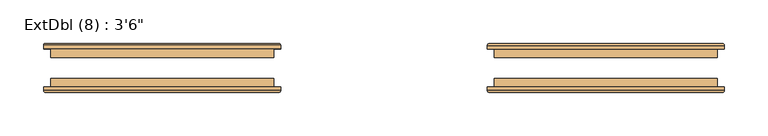
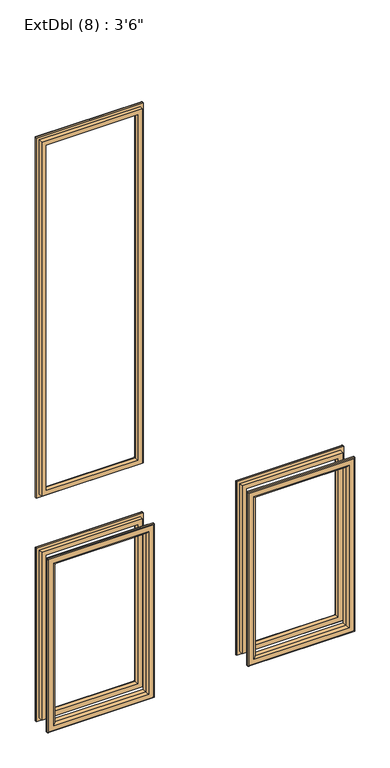
"""IFC4 building model written with IfcOpenShell, lengths in millimetres: door geometry."""

from ifc_helpers import new_model, si_unit, frame, origin, place, context, project, spatial, ellipse_curve, source, transform, mapped, element, save
from ifc_brep_helpers import plane_surface, cylinder_surface, advanced_brep


def door_55c03dfd(model_context):
    return source(origin(), model_context, "Body", "AdvancedBrep", [
        advanced_brep(
        [(-389.9, -29.8, 950.5), (-389.9, -33.8, 950.5), (-389.9, -33.8, 1916.5), (-389.9, -29.8, 1916.5), (-387.9, -27.8, 952.5), (-387.9, -27.8, 1914.5), (-369.9, -32.8, 970.5), (-374.9, -27.8, 965.5), (-374.9, -27.8, 1901.5), (-369.9, -32.8, 1896.5), (-369.9, -43.8, 970.5), (-369.9, -43.8, 1896.5), (-381.9, -33.8, 958.5), (-381.9, -43.8, 958.5), (-381.9, -43.8, 1908.5), (-381.9, -33.8, 1908.5), (-118.5, -33.8, 1916.5), (-118.5, -29.8, 1916.5), (-120.5, -27.8, 1914.5), (-133.5, -27.8, 1901.5), (-138.5, -32.8, 1896.5), (-138.5, -43.8, 1896.5), (-126.5, -43.8, 1908.5), (-126.5, -33.8, 1908.5), (-118.5, -33.8, 950.5), (-118.5, -29.8, 950.5), (-120.5, -27.8, 952.5), (-133.5, -27.8, 965.5), (-138.5, -32.8, 970.5), (-138.5, -43.8, 970.5), (-126.5, -43.8, 958.5), (-126.5, -33.8, 958.5)],
        [
            (0, 1),
            (1, 2),
            (2, 3),
            (3, 0),
            (4, 0, ellipse_curve(frame((-387.9, -29.8, 952.5), z_axis=(-0.7071067811865472, 0.0, 0.7071067811865479), x_axis=(-0.7071067811865479, 0.0, -0.707106781186547)), 2.8284271, 2.0)),
            (3, 5, ellipse_curve(frame((-387.9, -29.8, 1914.5), z_axis=(-0.7071067811865475, 0.0, -0.7071067811865475), x_axis=(0.7071067811865474, 0.0, -0.7071067811865476)), 2.8284271, 2.0)),
            (5, 4),
            (6, 7, ellipse_curve(frame((-374.9, -32.8, 965.5), z_axis=(-0.7071067811865472, 0.0, 0.7071067811865479), x_axis=(-0.7071067811865479, 0.0, -0.707106781186547)), 7.0710678, 5.0)),
            (7, 8),
            (8, 9, ellipse_curve(frame((-374.9, -32.8, 1901.5), z_axis=(-0.7071067811865475, 0.0, -0.7071067811865475), x_axis=(0.7071067811865474, 0.0, -0.7071067811865476)), 7.0710678, 5.0)),
            (9, 6),
            (10, 6),
            (9, 11),
            (11, 10),
            (12, 13),
            (13, 14),
            (14, 15),
            (15, 12),
            (2, 16),
            (16, 17),
            (17, 3),
            (17, 18, ellipse_curve(frame((-120.5, -29.8, 1914.5), z_axis=(-0.7071067811865475, 0.0, 0.7071067811865476), x_axis=(-0.7071067811865476, 0.0, -0.7071067811865475)), 2.8284271, 2.0)),
            (18, 5),
            (8, 19),
            (19, 20, ellipse_curve(frame((-133.5, -32.8, 1901.5), z_axis=(-0.7071067811865475, 0.0, 0.7071067811865476), x_axis=(-0.7071067811865476, 0.0, -0.7071067811865475)), 7.0710678, 5.0)),
            (20, 9),
            (20, 21),
            (21, 11),
            (14, 22),
            (22, 23),
            (23, 15),
            (16, 24),
            (24, 25),
            (25, 17),
            (25, 26, ellipse_curve(frame((-120.5, -29.8, 952.5), z_axis=(0.7071067811865478, 0.0, 0.7071067811865471), x_axis=(-0.707106781186547, 0.0, 0.707106781186548)), 2.8284271, 2.0)),
            (26, 18),
            (19, 27),
            (27, 28, ellipse_curve(frame((-133.5, -32.8, 965.5), z_axis=(0.7071067811865478, 0.0, 0.7071067811865471), x_axis=(-0.707106781186547, 0.0, 0.707106781186548)), 7.0710678, 5.0)),
            (28, 20),
            (28, 29),
            (29, 21),
            (22, 30),
            (30, 31),
            (31, 23),
            (24, 1),
            (0, 25),
            (4, 26),
            (7, 27),
            (6, 28),
            (10, 29),
            (13, 30),
            (12, 31),
        ],
        [
            plane_surface(frame((-389.9, -33.8, 950.5), z_axis=(-1.0, 0.0, 0.0), x_axis=(0.0, 0.0, 1.0))),
            cylinder_surface(frame((-387.9, -29.8, 958.5), z_axis=(0.0, 0.0, -1.0), x_axis=(-1.0, 0.0, 0.0)), 2.0),
            cylinder_surface(frame((-374.9, -32.8, 958.5), z_axis=(0.0, 0.0, -1.0), x_axis=(-1.0, 0.0, 0.0)), 5.0),
            plane_surface(frame((-369.9, -32.8, 970.5), z_axis=(1.0, 0.0, 0.0), x_axis=(0.0, 0.0, 1.0))),
            plane_surface(frame((-381.9, -43.8, 958.5), z_axis=(-1.0, 0.0, 0.0), x_axis=(0.0, 0.0, 1.0))),
            plane_surface(frame((-389.9, -33.8, 1916.5), z_axis=(0.0, 0.0, 1.0), x_axis=(1.0, 0.0, 0.0))),
            cylinder_surface(frame((-381.9, -29.8, 1914.5), z_axis=(-1.0, 0.0, 0.0), x_axis=(0.0, 0.0, 1.0)), 2.0),
            cylinder_surface(frame((-381.9, -32.8, 1901.5), z_axis=(-1.0, 0.0, 0.0), x_axis=(0.0, 0.0, 1.0)), 5.0),
            plane_surface(frame((-369.9, -32.8, 1896.5), z_axis=(0.0, 0.0, -1.0), x_axis=(1.0, 0.0, 0.0))),
            plane_surface(frame((-381.9, -43.8, 1908.5), z_axis=(0.0, 0.0, 1.0), x_axis=(1.0, 0.0, 0.0))),
            plane_surface(frame((-118.5, -33.8, 1916.5), z_axis=(1.0, 0.0, 0.0), x_axis=(0.0, 0.0, -1.0))),
            cylinder_surface(frame((-120.5, -29.8, 1908.5), z_axis=(0.0, 0.0, 1.0), x_axis=(1.0, 0.0, 0.0)), 2.0),
            cylinder_surface(frame((-133.5, -32.8, 1908.5), z_axis=(0.0, 0.0, 1.0), x_axis=(1.0, 0.0, 0.0)), 5.0),
            plane_surface(frame((-138.5, -32.8, 1896.5), z_axis=(-1.0, 0.0, 0.0), x_axis=(0.0, 0.0, -1.0))),
            plane_surface(frame((-126.5, -43.8, 1908.5), z_axis=(1.0, 0.0, 0.0), x_axis=(0.0, 0.0, -1.0))),
            plane_surface(frame((-118.5, -33.8, 950.5), z_axis=(0.0, 0.0, -1.0), x_axis=(-1.0, 0.0, 0.0))),
            cylinder_surface(frame((-126.5, -29.8, 952.5), z_axis=(1.0, 0.0, 0.0), x_axis=(0.0, 0.0, -1.0)), 2.0),
            plane_surface(frame((-120.5, -27.8, 952.5), z_axis=(0.0, 1.0, 0.0), x_axis=(-1.0, 0.0, 0.0))),
            cylinder_surface(frame((-126.5, -32.8, 965.5), z_axis=(1.0, 0.0, 0.0), x_axis=(0.0, 0.0, -1.0)), 5.0),
            plane_surface(frame((-138.5, -32.8, 970.5), z_axis=(0.0, 0.0, 1.0), x_axis=(-1.0, 0.0, 0.0))),
            plane_surface(frame((-138.5, -43.8, 970.5), z_axis=(0.0, -1.0, 0.0), x_axis=(-1.0, 0.0, 0.0))),
            plane_surface(frame((-126.5, -43.8, 958.5), z_axis=(0.0, 0.0, -1.0), x_axis=(-1.0, 0.0, 0.0))),
            plane_surface(frame((-126.5, -33.8, 958.5), z_axis=(0.0, -1.0, 0.0), x_axis=(-1.0, 0.0, 0.0))),
        ],
        [
            (0, [[1, 2, 3, 4]]),
            (1, [[5, -4, 6, 7]]),
            (2, [[8, 9, 10, 11]]),
            (3, [[12, -11, 13, 14]]),
            (4, [[15, 16, 17, 18]]),
            (5, [[-3, 19, 20, 21]]),
            (6, [[-6, -21, 22, 23]]),
            (7, [[-10, 24, 25, 26]]),
            (8, [[-13, -26, 27, 28]]),
            (9, [[-17, 29, 30, 31]]),
            (10, [[-20, 32, 33, 34]]),
            (11, [[-22, -34, 35, 36]]),
            (12, [[-25, 37, 38, 39]]),
            (13, [[-27, -39, 40, 41]]),
            (14, [[-30, 42, 43, 44]]),
            (15, [[-33, 45, -1, 46]]),
            (16, [[-35, -46, -5, 47]]),
            (17, [[-23, -36, -47, -7], [48, -37, -24, -9]]),
            (18, [[-38, -48, -8, 49]]),
            (19, [[-40, -49, -12, 50]]),
            (20, [[51, -42, -29, -16], [-28, -41, -50, -14]]),
            (21, [[-43, -51, -15, 52]]),
            (22, [[-45, -32, -19, -2], [-31, -44, -52, -18]]),
        ],
    ),
        advanced_brep(
        [(126.5, -43.8, 808.5), (126.5, -33.8, 808.5), (126.5, -33.8, 358.5), (126.5, -43.8, 358.5), (138.5, -32.8, 796.5), (138.5, -43.8, 796.5), (138.5, -43.8, 370.5), (138.5, -32.8, 370.5), (133.5, -27.8, 801.5), (133.5, -27.8, 365.5), (118.5, -29.8, 816.5), (120.5, -27.8, 814.5), (120.5, -27.8, 352.5), (118.5, -29.8, 350.5), (118.5, -33.8, 816.5), (118.5, -33.8, 350.5), (381.9, -33.8, 358.5), (381.9, -43.8, 358.5), (369.9, -43.8, 370.5), (369.9, -32.8, 370.5), (374.9, -27.8, 365.5), (387.9, -27.8, 352.5), (389.9, -29.8, 350.5), (389.9, -33.8, 350.5), (381.9, -33.8, 808.5), (381.9, -43.8, 808.5), (369.9, -43.8, 796.5), (369.9, -32.8, 796.5), (374.9, -27.8, 801.5), (387.9, -27.8, 814.5), (389.9, -29.8, 816.5), (389.9, -33.8, 816.5)],
        [
            (0, 1),
            (1, 2),
            (2, 3),
            (3, 0),
            (4, 5),
            (5, 6),
            (6, 7),
            (7, 4),
            (8, 4, ellipse_curve(frame((133.5, -32.8, 801.5), z_axis=(-0.7071067811865475, 0.0, -0.7071067811865475), x_axis=(-0.7071067811865474, 0.0, 0.7071067811865476)), 7.0710678, 5.0)),
            (7, 9, ellipse_curve(frame((133.5, -32.8, 365.5), z_axis=(-0.7071067811865475, 0.0, 0.7071067811865475), x_axis=(0.7071067811865474, 0.0, 0.7071067811865476)), 7.0710678, 5.0)),
            (9, 8),
            (10, 11, ellipse_curve(frame((120.5, -29.8, 814.5), z_axis=(-0.7071067811865475, 0.0, -0.7071067811865475), x_axis=(-0.7071067811865474, 0.0, 0.7071067811865476)), 2.8284271, 2.0)),
            (11, 12),
            (12, 13, ellipse_curve(frame((120.5, -29.8, 352.5), z_axis=(-0.7071067811865475, 0.0, 0.7071067811865475), x_axis=(0.7071067811865474, 0.0, 0.7071067811865476)), 2.8284271, 2.0)),
            (13, 10),
            (14, 10),
            (13, 15),
            (15, 14),
            (2, 16),
            (16, 17),
            (17, 3),
            (6, 18),
            (18, 19),
            (19, 7),
            (19, 20, ellipse_curve(frame((374.9, -32.8, 365.5), z_axis=(-0.7071067811865476, 0.0, -0.7071067811865475), x_axis=(-0.7071067811865475, 0.0, 0.7071067811865476)), 7.0710678, 5.0)),
            (20, 9),
            (12, 21),
            (21, 22, ellipse_curve(frame((387.9, -29.8, 352.5), z_axis=(-0.7071067811865476, 0.0, -0.7071067811865475), x_axis=(-0.7071067811865475, 0.0, 0.7071067811865476)), 2.8284271, 2.0)),
            (22, 13),
            (22, 23),
            (23, 15),
            (16, 24),
            (24, 25),
            (25, 17),
            (18, 26),
            (26, 27),
            (27, 19),
            (27, 28, ellipse_curve(frame((374.9, -32.8, 801.5), z_axis=(0.7071067811865475, 0.0, -0.7071067811865476), x_axis=(-0.7071067811865476, 0.0, -0.7071067811865475)), 7.0710678, 5.0)),
            (28, 20),
            (21, 29),
            (29, 30, ellipse_curve(frame((387.9, -29.8, 814.5), z_axis=(0.7071067811865475, 0.0, -0.7071067811865476), x_axis=(-0.7071067811865476, 0.0, -0.7071067811865475)), 2.8284271, 2.0)),
            (30, 22),
            (30, 31),
            (31, 23),
            (31, 14),
            (1, 24),
            (0, 25),
            (5, 26),
            (4, 27),
            (8, 28),
            (11, 29),
            (10, 30),
        ],
        [
            plane_surface(frame((126.5, -33.8, 808.5), z_axis=(-1.0, 0.0, 0.0), x_axis=(0.0, 0.0, -1.0))),
            plane_surface(frame((138.5, -43.8, 796.5), z_axis=(1.0, 0.0, 0.0), x_axis=(0.0, 0.0, -1.0))),
            cylinder_surface(frame((133.5, -32.8, 808.5), z_axis=(0.0, 0.0, 1.0), x_axis=(-1.0, 0.0, 0.0)), 5.0),
            cylinder_surface(frame((120.5, -29.8, 808.5), z_axis=(0.0, 0.0, 1.0), x_axis=(-1.0, 0.0, 0.0)), 2.0),
            plane_surface(frame((118.5, -29.8, 816.5), z_axis=(-1.0, 0.0, 0.0), x_axis=(0.0, 0.0, -1.0))),
            plane_surface(frame((126.5, -33.8, 358.5), z_axis=(0.0, 0.0, -1.0), x_axis=(1.0, 0.0, 0.0))),
            plane_surface(frame((138.5, -43.8, 370.5), z_axis=(0.0, 0.0, 1.0), x_axis=(1.0, 0.0, 0.0))),
            cylinder_surface(frame((126.5, -32.8, 365.5), z_axis=(-1.0, 0.0, 0.0), x_axis=(0.0, 0.0, -1.0)), 5.0),
            cylinder_surface(frame((126.5, -29.8, 352.5), z_axis=(-1.0, 0.0, 0.0), x_axis=(0.0, 0.0, -1.0)), 2.0),
            plane_surface(frame((118.5, -29.8, 350.5), z_axis=(0.0, 0.0, -1.0), x_axis=(1.0, 0.0, 0.0))),
            plane_surface(frame((381.9, -33.8, 358.5), z_axis=(1.0, 0.0, 0.0), x_axis=(0.0, 0.0, 1.0))),
            plane_surface(frame((369.9, -43.8, 370.5), z_axis=(-1.0, 0.0, 0.0), x_axis=(0.0, 0.0, 1.0))),
            cylinder_surface(frame((374.9, -32.8, 358.5), z_axis=(0.0, 0.0, -1.0), x_axis=(1.0, 0.0, 0.0)), 5.0),
            cylinder_surface(frame((387.9, -29.8, 358.5), z_axis=(0.0, 0.0, -1.0), x_axis=(1.0, 0.0, 0.0)), 2.0),
            plane_surface(frame((389.9, -29.8, 350.5), z_axis=(1.0, 0.0, 0.0), x_axis=(0.0, 0.0, 1.0))),
            plane_surface(frame((389.9, -33.8, 816.5), z_axis=(0.0, -1.0, 0.0), x_axis=(-1.0, 0.0, 0.0))),
            plane_surface(frame((381.9, -33.8, 808.5), z_axis=(0.0, 0.0, 1.0), x_axis=(-1.0, 0.0, 0.0))),
            plane_surface(frame((381.9, -43.8, 808.5), z_axis=(0.0, -1.0, 0.0), x_axis=(-1.0, 0.0, 0.0))),
            plane_surface(frame((369.9, -43.8, 796.5), z_axis=(0.0, 0.0, -1.0), x_axis=(-1.0, 0.0, 0.0))),
            cylinder_surface(frame((381.9, -32.8, 801.5), z_axis=(1.0, 0.0, 0.0), x_axis=(0.0, 0.0, 1.0)), 5.0),
            plane_surface(frame((374.9, -27.8, 801.5), z_axis=(0.0, 1.0, 0.0), x_axis=(-1.0, 0.0, 0.0))),
            cylinder_surface(frame((381.9, -29.8, 814.5), z_axis=(1.0, 0.0, 0.0), x_axis=(0.0, 0.0, 1.0)), 2.0),
            plane_surface(frame((389.9, -29.8, 816.5), z_axis=(0.0, 0.0, 1.0), x_axis=(-1.0, 0.0, 0.0))),
        ],
        [
            (0, [[1, 2, 3, 4]]),
            (1, [[5, 6, 7, 8]]),
            (2, [[9, -8, 10, 11]]),
            (3, [[12, 13, 14, 15]]),
            (4, [[16, -15, 17, 18]]),
            (5, [[-3, 19, 20, 21]]),
            (6, [[-7, 22, 23, 24]]),
            (7, [[-10, -24, 25, 26]]),
            (8, [[-14, 27, 28, 29]]),
            (9, [[-17, -29, 30, 31]]),
            (10, [[-20, 32, 33, 34]]),
            (11, [[-23, 35, 36, 37]]),
            (12, [[-25, -37, 38, 39]]),
            (13, [[-28, 40, 41, 42]]),
            (14, [[-30, -42, 43, 44]]),
            (15, [[-31, -44, 45, -18], [46, -32, -19, -2]]),
            (16, [[-33, -46, -1, 47]]),
            (17, [[-21, -34, -47, -4], [48, -35, -22, -6]]),
            (18, [[-36, -48, -5, 49]]),
            (19, [[-38, -49, -9, 50]]),
            (20, [[51, -40, -27, -13], [-26, -39, -50, -11]]),
            (21, [[-41, -51, -12, 52]]),
            (22, [[-43, -52, -16, -45]]),
        ],
    ),
        advanced_brep(
        [(381.9, -67.8, 808.5), (381.9, -77.8, 808.5), (381.9, -77.8, 358.5), (381.9, -67.8, 358.5), (369.9, -78.8, 796.5), (369.9, -67.8, 796.5), (369.9, -67.8, 370.5), (369.9, -78.8, 370.5), (374.9, -83.8, 801.5), (374.9, -83.8, 365.5), (389.9, -81.8, 816.5), (387.9, -83.8, 814.5), (387.9, -83.8, 352.5), (389.9, -81.8, 350.5), (389.9, -77.8, 816.5), (389.9, -77.8, 350.5), (126.5, -77.8, 358.5), (126.5, -67.8, 358.5), (138.5, -67.8, 370.5), (138.5, -78.8, 370.5), (133.5, -83.8, 365.5), (120.5, -83.8, 352.5), (118.5, -81.8, 350.5), (118.5, -77.8, 350.5), (126.5, -77.8, 808.5), (126.5, -67.8, 808.5), (138.5, -67.8, 796.5), (138.5, -78.8, 796.5), (133.5, -83.8, 801.5), (120.5, -83.8, 814.5), (118.5, -81.8, 816.5), (118.5, -77.8, 816.5)],
        [
            (0, 1),
            (1, 2),
            (2, 3),
            (3, 0),
            (4, 5),
            (5, 6),
            (6, 7),
            (7, 4),
            (8, 4, ellipse_curve(frame((374.9, -78.8, 801.5), z_axis=(0.707106781186552, 0.0, -0.707106781186543), x_axis=(0.7071067811865429, 0.0, 0.707106781186552)), 7.0710678, 5.0)),
            (7, 9, ellipse_curve(frame((374.9, -78.8, 365.5), z_axis=(0.707106781186543, 0.0, 0.707106781186552), x_axis=(-0.707106781186552, 0.0, 0.707106781186543)), 7.0710678, 5.0)),
            (9, 8),
            (10, 11, ellipse_curve(frame((387.9, -81.8, 814.5), z_axis=(0.707106781186552, 0.0, -0.707106781186543), x_axis=(0.7071067811865429, 0.0, 0.707106781186552)), 2.8284271, 2.0)),
            (11, 12),
            (12, 13, ellipse_curve(frame((387.9, -81.8, 352.5), z_axis=(0.707106781186543, 0.0, 0.707106781186552), x_axis=(-0.707106781186552, 0.0, 0.707106781186543)), 2.8284271, 2.0)),
            (13, 10),
            (14, 10),
            (13, 15),
            (15, 14),
            (2, 16),
            (16, 17),
            (17, 3),
            (6, 18),
            (18, 19),
            (19, 7),
            (19, 20, ellipse_curve(frame((133.5, -78.8, 365.5), z_axis=(0.707106781186552, 0.0, -0.7071067811865431), x_axis=(0.7071067811865429, 0.0, 0.707106781186552)), 7.0710678, 5.0)),
            (20, 9),
            (12, 21),
            (21, 22, ellipse_curve(frame((120.5, -81.8, 352.5), z_axis=(0.707106781186552, 0.0, -0.7071067811865431), x_axis=(0.7071067811865429, 0.0, 0.707106781186552)), 2.8284271, 2.0)),
            (22, 13),
            (22, 23),
            (23, 15),
            (16, 24),
            (24, 25),
            (25, 17),
            (18, 26),
            (26, 27),
            (27, 19),
            (27, 28, ellipse_curve(frame((133.5, -78.8, 801.5), z_axis=(-0.707106781186543, 0.0, -0.7071067811865519), x_axis=(0.7071067811865517, 0.0, -0.7071067811865432)), 7.0710678, 5.0)),
            (28, 20),
            (21, 29),
            (29, 30, ellipse_curve(frame((120.5, -81.8, 814.5), z_axis=(-0.707106781186543, 0.0, -0.7071067811865519), x_axis=(0.7071067811865517, 0.0, -0.7071067811865432)), 2.8284271, 2.0)),
            (30, 22),
            (30, 31),
            (31, 23),
            (31, 14),
            (1, 24),
            (0, 25),
            (5, 26),
            (4, 27),
            (8, 28),
            (11, 29),
            (10, 30),
        ],
        [
            plane_surface(frame((381.9, -77.8, 808.5), z_axis=(1.0, 0.0, 0.0), x_axis=(0.0, 0.0, -1.0))),
            plane_surface(frame((369.9, -67.8, 796.5), z_axis=(-1.0, 0.0, 0.0), x_axis=(0.0, 0.0, -1.0))),
            cylinder_surface(frame((374.9, -78.8, 808.5), z_axis=(0.0, 0.0, 1.0), x_axis=(1.0, 0.0, 0.0)), 5.0),
            cylinder_surface(frame((387.9, -81.8, 808.5), z_axis=(0.0, 0.0, 1.0), x_axis=(1.0, 0.0, 0.0)), 2.0),
            plane_surface(frame((389.9, -81.8, 816.5), z_axis=(1.0, 0.0, 0.0), x_axis=(0.0, 0.0, -1.0))),
            plane_surface(frame((381.9, -77.8, 358.5), z_axis=(0.0, 0.0, -1.0), x_axis=(-1.0, 0.0, 0.0))),
            plane_surface(frame((369.9, -67.8, 370.5), z_axis=(0.0, 0.0, 1.0), x_axis=(-1.0, 0.0, 0.0))),
            cylinder_surface(frame((381.9, -78.8, 365.5), z_axis=(1.0, 0.0, 0.0), x_axis=(0.0, 0.0, -1.0)), 5.0),
            cylinder_surface(frame((381.9, -81.8, 352.5), z_axis=(1.0, 0.0, 0.0), x_axis=(0.0, 0.0, -1.0)), 2.0),
            plane_surface(frame((389.9, -81.8, 350.5), z_axis=(0.0, 0.0, -1.0), x_axis=(-1.0, 0.0, 0.0))),
            plane_surface(frame((126.5, -77.8, 358.5), z_axis=(-1.0, 0.0, 0.0), x_axis=(0.0, 0.0, 1.0))),
            plane_surface(frame((138.5, -67.8, 370.5), z_axis=(1.0, 0.0, 0.0), x_axis=(0.0, 0.0, 1.0))),
            cylinder_surface(frame((133.5, -78.8, 358.5), z_axis=(0.0, 0.0, -1.0), x_axis=(-1.0, 0.0, 0.0)), 5.0),
            cylinder_surface(frame((120.5, -81.8, 358.5), z_axis=(0.0, 0.0, -1.0), x_axis=(-1.0, 0.0, 0.0)), 2.0),
            plane_surface(frame((118.5, -81.8, 350.5), z_axis=(-1.0, 0.0, 0.0), x_axis=(0.0, 0.0, 1.0))),
            plane_surface(frame((118.5, -77.8, 816.5), z_axis=(0.0, 1.0, 0.0), x_axis=(1.0, 0.0, 0.0))),
            plane_surface(frame((126.5, -77.8, 808.5), z_axis=(0.0, 0.0, 1.0), x_axis=(1.0, 0.0, 0.0))),
            plane_surface(frame((126.5, -67.8, 808.5), z_axis=(0.0, 1.0, 0.0), x_axis=(1.0, 0.0, 0.0))),
            plane_surface(frame((138.5, -67.8, 796.5), z_axis=(0.0, 0.0, -1.0), x_axis=(1.0, 0.0, 0.0))),
            cylinder_surface(frame((126.5, -78.8, 801.5), z_axis=(-1.0, 0.0, 0.0), x_axis=(0.0, 0.0, 1.0)), 5.0),
            plane_surface(frame((133.5, -83.8, 801.5), z_axis=(0.0, -1.0, 0.0), x_axis=(1.0, 0.0, 0.0))),
            cylinder_surface(frame((126.5, -81.8, 814.5), z_axis=(-1.0, 0.0, 0.0), x_axis=(0.0, 0.0, 1.0)), 2.0),
            plane_surface(frame((118.5, -81.8, 816.5), z_axis=(0.0, 0.0, 1.0), x_axis=(1.0, 0.0, 0.0))),
        ],
        [
            (0, [[1, 2, 3, 4]]),
            (1, [[5, 6, 7, 8]]),
            (2, [[9, -8, 10, 11]]),
            (3, [[12, 13, 14, 15]]),
            (4, [[16, -15, 17, 18]]),
            (5, [[-3, 19, 20, 21]]),
            (6, [[-7, 22, 23, 24]]),
            (7, [[-10, -24, 25, 26]]),
            (8, [[-14, 27, 28, 29]]),
            (9, [[-17, -29, 30, 31]]),
            (10, [[-20, 32, 33, 34]]),
            (11, [[-23, 35, 36, 37]]),
            (12, [[-25, -37, 38, 39]]),
            (13, [[-28, 40, 41, 42]]),
            (14, [[-30, -42, 43, 44]]),
            (15, [[-31, -44, 45, -18], [46, -32, -19, -2]]),
            (16, [[-33, -46, -1, 47]]),
            (17, [[-21, -34, -47, -4], [48, -35, -22, -6]]),
            (18, [[-36, -48, -5, 49]]),
            (19, [[-38, -49, -9, 50]]),
            (20, [[51, -40, -27, -13], [-26, -39, -50, -11]]),
            (21, [[-41, -51, -12, 52]]),
            (22, [[-43, -52, -16, -45]]),
        ],
    ),
        advanced_brep(
        [(-381.9, -43.8, 808.5), (-381.9, -33.8, 808.5), (-381.9, -33.8, 358.5), (-381.9, -43.8, 358.5), (-369.9, -32.8, 796.5), (-369.9, -43.8, 796.5), (-369.9, -43.8, 370.5), (-369.9, -32.8, 370.5), (-374.9, -27.8, 801.5), (-374.9, -27.8, 365.5), (-389.9, -29.8, 816.5), (-387.9, -27.8, 814.5), (-387.9, -27.8, 352.5), (-389.9, -29.8, 350.5), (-389.9, -33.8, 816.5), (-389.9, -33.8, 350.5), (-126.5, -33.8, 358.5), (-126.5, -43.8, 358.5), (-138.5, -43.8, 370.5), (-138.5, -32.8, 370.5), (-133.5, -27.8, 365.5), (-120.5, -27.8, 352.5), (-118.5, -29.8, 350.5), (-118.5, -33.8, 350.5), (-126.5, -33.8, 808.5), (-126.5, -43.8, 808.5), (-138.5, -43.8, 796.5), (-138.5, -32.8, 796.5), (-133.5, -27.8, 801.5), (-120.5, -27.8, 814.5), (-118.5, -29.8, 816.5), (-118.5, -33.8, 816.5)],
        [
            (0, 1),
            (1, 2),
            (2, 3),
            (3, 0),
            (4, 5),
            (5, 6),
            (6, 7),
            (7, 4),
            (8, 4, ellipse_curve(frame((-374.9, -32.8, 801.5), z_axis=(-0.7071067811865477, 0.0, -0.7071067811865474), x_axis=(-0.7071067811865474, 0.0, 0.7071067811865477)), 7.0710678, 5.0)),
            (7, 9, ellipse_curve(frame((-374.9, -32.8, 365.5), z_axis=(-0.7071067811865475, 0.0, 0.7071067811865475), x_axis=(0.7071067811865474, 0.0, 0.7071067811865476)), 7.0710678, 5.0)),
            (9, 8),
            (10, 11, ellipse_curve(frame((-387.9, -29.8, 814.5), z_axis=(-0.7071067811865477, 0.0, -0.7071067811865474), x_axis=(-0.7071067811865474, 0.0, 0.7071067811865477)), 2.8284271, 2.0)),
            (11, 12),
            (12, 13, ellipse_curve(frame((-387.9, -29.8, 352.5), z_axis=(-0.7071067811865475, 0.0, 0.7071067811865475), x_axis=(0.7071067811865474, 0.0, 0.7071067811865476)), 2.8284271, 2.0)),
            (13, 10),
            (14, 10),
            (13, 15),
            (15, 14),
            (2, 16),
            (16, 17),
            (17, 3),
            (6, 18),
            (18, 19),
            (19, 7),
            (19, 20, ellipse_curve(frame((-133.5, -32.8, 365.5), z_axis=(-0.7071067811865475, 0.0, -0.7071067811865475), x_axis=(-0.7071067811865476, 0.0, 0.7071067811865474)), 7.0710678, 5.0)),
            (20, 9),
            (12, 21),
            (21, 22, ellipse_curve(frame((-120.5, -29.8, 352.5), z_axis=(-0.7071067811865475, 0.0, -0.7071067811865475), x_axis=(-0.7071067811865476, 0.0, 0.7071067811865474)), 2.8284271, 2.0)),
            (22, 13),
            (22, 23),
            (23, 15),
            (16, 24),
            (24, 25),
            (25, 17),
            (18, 26),
            (26, 27),
            (27, 19),
            (27, 28, ellipse_curve(frame((-133.5, -32.8, 801.5), z_axis=(0.7071067811865474, 0.0, -0.7071067811865477), x_axis=(-0.7071067811865477, 0.0, -0.7071067811865474)), 7.0710678, 5.0)),
            (28, 20),
            (21, 29),
            (29, 30, ellipse_curve(frame((-120.5, -29.8, 814.5), z_axis=(0.7071067811865474, 0.0, -0.7071067811865477), x_axis=(-0.7071067811865477, 0.0, -0.7071067811865474)), 2.8284271, 2.0)),
            (30, 22),
            (30, 31),
            (31, 23),
            (31, 14),
            (1, 24),
            (0, 25),
            (5, 26),
            (4, 27),
            (8, 28),
            (11, 29),
            (10, 30),
        ],
        [
            plane_surface(frame((-381.9, -33.8, 808.5), z_axis=(-1.0, 0.0, 0.0), x_axis=(0.0, 0.0, -1.0))),
            plane_surface(frame((-369.9, -43.8, 796.5), z_axis=(1.0, 0.0, 0.0), x_axis=(0.0, 0.0, -1.0))),
            cylinder_surface(frame((-374.9, -32.8, 808.5), z_axis=(0.0, 0.0, 1.0), x_axis=(-1.0, 0.0, 0.0)), 5.0),
            cylinder_surface(frame((-387.9, -29.8, 808.5), z_axis=(0.0, 0.0, 1.0), x_axis=(-1.0, 0.0, 0.0)), 2.0),
            plane_surface(frame((-389.9, -29.8, 816.5), z_axis=(-1.0, 0.0, 0.0), x_axis=(0.0, 0.0, -1.0))),
            plane_surface(frame((-381.9, -33.8, 358.5), z_axis=(0.0, 0.0, -1.0), x_axis=(1.0, 0.0, 0.0))),
            plane_surface(frame((-369.9, -43.8, 370.5), z_axis=(0.0, 0.0, 1.0), x_axis=(1.0, 0.0, 0.0))),
            cylinder_surface(frame((-381.9, -32.8, 365.5), z_axis=(-1.0, 0.0, 0.0), x_axis=(0.0, 0.0, -1.0)), 5.0),
            cylinder_surface(frame((-381.9, -29.8, 352.5), z_axis=(-1.0, 0.0, 0.0), x_axis=(0.0, 0.0, -1.0)), 2.0),
            plane_surface(frame((-389.9, -29.8, 350.5), z_axis=(0.0, 0.0, -1.0), x_axis=(1.0, 0.0, 0.0))),
            plane_surface(frame((-126.5, -33.8, 358.5), z_axis=(1.0, 0.0, 0.0), x_axis=(0.0, 0.0, 1.0))),
            plane_surface(frame((-138.5, -43.8, 370.5), z_axis=(-1.0, 0.0, 0.0), x_axis=(0.0, 0.0, 1.0))),
            cylinder_surface(frame((-133.5, -32.8, 358.5), z_axis=(0.0, 0.0, -1.0), x_axis=(1.0, 0.0, 0.0)), 5.0),
            cylinder_surface(frame((-120.5, -29.8, 358.5), z_axis=(0.0, 0.0, -1.0), x_axis=(1.0, 0.0, 0.0)), 2.0),
            plane_surface(frame((-118.5, -29.8, 350.5), z_axis=(1.0, 0.0, 0.0), x_axis=(0.0, 0.0, 1.0))),
            plane_surface(frame((-118.5, -33.8, 816.5), z_axis=(0.0, -1.0, 0.0), x_axis=(-1.0, 0.0, 0.0))),
            plane_surface(frame((-126.5, -33.8, 808.5), z_axis=(0.0, 0.0, 1.0), x_axis=(-1.0, 0.0, 0.0))),
            plane_surface(frame((-126.5, -43.8, 808.5), z_axis=(0.0, -1.0, 0.0), x_axis=(-1.0, 0.0, 0.0))),
            plane_surface(frame((-138.5, -43.8, 796.5), z_axis=(0.0, 0.0, -1.0), x_axis=(-1.0, 0.0, 0.0))),
            cylinder_surface(frame((-126.5, -32.8, 801.5), z_axis=(1.0, 0.0, 0.0), x_axis=(0.0, 0.0, 1.0)), 5.0),
            plane_surface(frame((-133.5, -27.8, 801.5), z_axis=(0.0, 1.0, 0.0), x_axis=(-1.0, 0.0, 0.0))),
            cylinder_surface(frame((-126.5, -29.8, 814.5), z_axis=(1.0, 0.0, 0.0), x_axis=(0.0, 0.0, 1.0)), 2.0),
            plane_surface(frame((-118.5, -29.8, 816.5), z_axis=(0.0, 0.0, 1.0), x_axis=(-1.0, 0.0, 0.0))),
        ],
        [
            (0, [[1, 2, 3, 4]]),
            (1, [[5, 6, 7, 8]]),
            (2, [[9, -8, 10, 11]]),
            (3, [[12, 13, 14, 15]]),
            (4, [[16, -15, 17, 18]]),
            (5, [[-3, 19, 20, 21]]),
            (6, [[-7, 22, 23, 24]]),
            (7, [[-10, -24, 25, 26]]),
            (8, [[-14, 27, 28, 29]]),
            (9, [[-17, -29, 30, 31]]),
            (10, [[-20, 32, 33, 34]]),
            (11, [[-23, 35, 36, 37]]),
            (12, [[-25, -37, 38, 39]]),
            (13, [[-28, 40, 41, 42]]),
            (14, [[-30, -42, 43, 44]]),
            (15, [[-31, -44, 45, -18], [46, -32, -19, -2]]),
            (16, [[-33, -46, -1, 47]]),
            (17, [[-21, -34, -47, -4], [48, -35, -22, -6]]),
            (18, [[-36, -48, -5, 49]]),
            (19, [[-38, -49, -9, 50]]),
            (20, [[51, -40, -27, -13], [-26, -39, -50, -11]]),
            (21, [[-41, -51, -12, 52]]),
            (22, [[-43, -52, -16, -45]]),
        ],
    ),
        advanced_brep(
        [(-126.5, -67.8, 808.5), (-126.5, -77.8, 808.5), (-126.5, -77.8, 358.5), (-126.5, -67.8, 358.5), (-138.5, -78.8, 796.5), (-138.5, -67.8, 796.5), (-138.5, -67.8, 370.5), (-138.5, -78.8, 370.5), (-133.5, -83.8, 801.5), (-133.5, -83.8, 365.5), (-118.5, -81.8, 816.5), (-120.5, -83.8, 814.5), (-120.5, -83.8, 352.5), (-118.5, -81.8, 350.5), (-118.5, -77.8, 816.5), (-118.5, -77.8, 350.5), (-381.9, -77.8, 358.5), (-381.9, -67.8, 358.5), (-369.9, -67.8, 370.5), (-369.9, -78.8, 370.5), (-374.9, -83.8, 365.5), (-387.9, -83.8, 352.5), (-389.9, -81.8, 350.5), (-389.9, -77.8, 350.5), (-381.9, -77.8, 808.5), (-381.9, -67.8, 808.5), (-369.9, -67.8, 796.5), (-369.9, -78.8, 796.5), (-374.9, -83.8, 801.5), (-387.9, -83.8, 814.5), (-389.9, -81.8, 816.5), (-389.9, -77.8, 816.5)],
        [
            (0, 1),
            (1, 2),
            (2, 3),
            (3, 0),
            (4, 5),
            (5, 6),
            (6, 7),
            (7, 4),
            (8, 4, ellipse_curve(frame((-133.5, -78.8, 801.5), z_axis=(0.707106781186552, 0.0, -0.7071067811865429), x_axis=(0.7071067811865428, 0.0, 0.7071067811865521)), 7.0710678, 5.0)),
            (7, 9, ellipse_curve(frame((-133.5, -78.8, 365.5), z_axis=(0.7071067811865429, 0.0, 0.707106781186552), x_axis=(-0.707106781186552, 0.0, 0.707106781186543)), 7.0710678, 5.0)),
            (9, 8),
            (10, 11, ellipse_curve(frame((-120.5, -81.8, 814.5), z_axis=(0.707106781186552, 0.0, -0.7071067811865429), x_axis=(0.7071067811865428, 0.0, 0.7071067811865521)), 2.8284271, 2.0)),
            (11, 12),
            (12, 13, ellipse_curve(frame((-120.5, -81.8, 352.5), z_axis=(0.7071067811865429, 0.0, 0.707106781186552), x_axis=(-0.707106781186552, 0.0, 0.707106781186543)), 2.8284271, 2.0)),
            (13, 10),
            (14, 10),
            (13, 15),
            (15, 14),
            (2, 16),
            (16, 17),
            (17, 3),
            (6, 18),
            (18, 19),
            (19, 7),
            (19, 20, ellipse_curve(frame((-374.9, -78.8, 365.5), z_axis=(0.7071067811865521, 0.0, -0.7071067811865428), x_axis=(0.7071067811865429, 0.0, 0.707106781186552)), 7.0710678, 5.0)),
            (20, 9),
            (12, 21),
            (21, 22, ellipse_curve(frame((-387.9, -81.8, 352.5), z_axis=(0.7071067811865521, 0.0, -0.7071067811865428), x_axis=(0.7071067811865429, 0.0, 0.707106781186552)), 2.8284271, 2.0)),
            (22, 13),
            (22, 23),
            (23, 15),
            (16, 24),
            (24, 25),
            (25, 17),
            (18, 26),
            (26, 27),
            (27, 19),
            (27, 28, ellipse_curve(frame((-374.9, -78.8, 801.5), z_axis=(-0.7071067811865429, 0.0, -0.7071067811865521), x_axis=(0.7071067811865521, 0.0, -0.7071067811865429)), 7.0710678, 5.0)),
            (28, 20),
            (21, 29),
            (29, 30, ellipse_curve(frame((-387.9, -81.8, 814.5), z_axis=(-0.7071067811865429, 0.0, -0.7071067811865521), x_axis=(0.7071067811865521, 0.0, -0.7071067811865429)), 2.8284271, 2.0)),
            (30, 22),
            (30, 31),
            (31, 23),
            (31, 14),
            (1, 24),
            (0, 25),
            (5, 26),
            (4, 27),
            (8, 28),
            (11, 29),
            (10, 30),
        ],
        [
            plane_surface(frame((-126.5, -77.8, 808.5), z_axis=(1.0, 0.0, 0.0), x_axis=(0.0, 0.0, -1.0))),
            plane_surface(frame((-138.5, -67.8, 796.5), z_axis=(-1.0, 0.0, 0.0), x_axis=(0.0, 0.0, -1.0))),
            cylinder_surface(frame((-133.5, -78.8, 808.5), z_axis=(0.0, 0.0, 1.0), x_axis=(1.0, 0.0, 0.0)), 5.0),
            cylinder_surface(frame((-120.5, -81.8, 808.5), z_axis=(0.0, 0.0, 1.0), x_axis=(1.0, 0.0, 0.0)), 2.0),
            plane_surface(frame((-118.5, -81.8, 816.5), z_axis=(1.0, 0.0, 0.0), x_axis=(0.0, 0.0, -1.0))),
            plane_surface(frame((-126.5, -77.8, 358.5), z_axis=(0.0, 0.0, -1.0), x_axis=(-1.0, 0.0, 0.0))),
            plane_surface(frame((-138.5, -67.8, 370.5), z_axis=(0.0, 0.0, 1.0), x_axis=(-1.0, 0.0, 0.0))),
            cylinder_surface(frame((-126.5, -78.8, 365.5), z_axis=(1.0, 0.0, 0.0), x_axis=(0.0, 0.0, -1.0)), 5.0),
            cylinder_surface(frame((-126.5, -81.8, 352.5), z_axis=(1.0, 0.0, 0.0), x_axis=(0.0, 0.0, -1.0)), 2.0),
            plane_surface(frame((-118.5, -81.8, 350.5), z_axis=(0.0, 0.0, -1.0), x_axis=(-1.0, 0.0, 0.0))),
            plane_surface(frame((-381.9, -77.8, 358.5), z_axis=(-1.0, 0.0, 0.0), x_axis=(0.0, 0.0, 1.0))),
            plane_surface(frame((-369.9, -67.8, 370.5), z_axis=(1.0, 0.0, 0.0), x_axis=(0.0, 0.0, 1.0))),
            cylinder_surface(frame((-374.9, -78.8, 358.5), z_axis=(0.0, 0.0, -1.0), x_axis=(-1.0, 0.0, 0.0)), 5.0),
            cylinder_surface(frame((-387.9, -81.8, 358.5), z_axis=(0.0, 0.0, -1.0), x_axis=(-1.0, 0.0, 0.0)), 2.0),
            plane_surface(frame((-389.9, -81.8, 350.5), z_axis=(-1.0, 0.0, 0.0), x_axis=(0.0, 0.0, 1.0))),
            plane_surface(frame((-389.9, -77.8, 816.5), z_axis=(0.0, 1.0, 0.0), x_axis=(1.0, 0.0, 0.0))),
            plane_surface(frame((-381.9, -77.8, 808.5), z_axis=(0.0, 0.0, 1.0), x_axis=(1.0, 0.0, 0.0))),
            plane_surface(frame((-381.9, -67.8, 808.5), z_axis=(0.0, 1.0, 0.0), x_axis=(1.0, 0.0, 0.0))),
            plane_surface(frame((-369.9, -67.8, 796.5), z_axis=(0.0, 0.0, -1.0), x_axis=(1.0, 0.0, 0.0))),
            cylinder_surface(frame((-381.9, -78.8, 801.5), z_axis=(-1.0, 0.0, 0.0), x_axis=(0.0, 0.0, 1.0)), 5.0),
            plane_surface(frame((-374.9, -83.8, 801.5), z_axis=(0.0, -1.0, 0.0), x_axis=(1.0, 0.0, 0.0))),
            cylinder_surface(frame((-381.9, -81.8, 814.5), z_axis=(-1.0, 0.0, 0.0), x_axis=(0.0, 0.0, 1.0)), 2.0),
            plane_surface(frame((-389.9, -81.8, 816.5), z_axis=(0.0, 0.0, 1.0), x_axis=(1.0, 0.0, 0.0))),
        ],
        [
            (0, [[1, 2, 3, 4]]),
            (1, [[5, 6, 7, 8]]),
            (2, [[9, -8, 10, 11]]),
            (3, [[12, 13, 14, 15]]),
            (4, [[16, -15, 17, 18]]),
            (5, [[-3, 19, 20, 21]]),
            (6, [[-7, 22, 23, 24]]),
            (7, [[-10, -24, 25, 26]]),
            (8, [[-14, 27, 28, 29]]),
            (9, [[-17, -29, 30, 31]]),
            (10, [[-20, 32, 33, 34]]),
            (11, [[-23, 35, 36, 37]]),
            (12, [[-25, -37, 38, 39]]),
            (13, [[-28, 40, 41, 42]]),
            (14, [[-30, -42, 43, 44]]),
            (15, [[-31, -44, 45, -18], [46, -32, -19, -2]]),
            (16, [[-33, -46, -1, 47]]),
            (17, [[-21, -34, -47, -4], [48, -35, -22, -6]]),
            (18, [[-36, -48, -5, 49]]),
            (19, [[-38, -49, -9, 50]]),
            (20, [[51, -40, -27, -13], [-26, -39, -50, -11]]),
            (21, [[-41, -51, -12, 52]]),
            (22, [[-43, -52, -16, -45]]),
        ],
    ),
    ])


if __name__ == "__main__":
    model = new_model("IFC4")
    model_context = context("Model", 3, world=origin())
    ifc_project = project(units=[si_unit("LENGTHUNIT", "METRE", prefix="MILLI")], contexts=[model_context])
    site = spatial("IfcSite", under=ifc_project)
    building = spatial("IfcBuilding", under=site)
    placement = place(None, origin())
    door_shape = door_55c03dfd(model_context)
    element("IfcDoor", 1, ObjectType="ExtDbl (8) : 3'6\"", at=placement, inside=building, context=model_context, shape_type="MappedRepresentation", body=[
        mapped(door_shape, transform((0.0, 0.0, 0.0), x_axis=(1.0, 0.0, 0.0), y_axis=(0.0, 1.0, 0.0), z_axis=(0.0, 0.0, 1.0))),
    ])
    save(model, "model.ifc")

# Revit data of these elements
# Type "ExtDbl (8) : 3'6\""
#   Type Mark = "14"
#   Operation = "DoubleDoorSingleSwing"
#   Keynote = "L20"
#   Wrap Layers (Int) from Ext = 0' - 6.98819"
#   Wrap Layers (Ext) from Ext = 0' - 4.03543"
#   Top of Lock Rail = 2' - 11.43307"
#   Thickness = 0' - 1.73228"
#   Stile Shutting = 0' - 4.92126"
#   Stile - Top Rail = 0' - 5.90551"
#   Stile - Lock Rail = 0' - 5.90551"
#   Stile - Hanging = 0' - 3.93701"
#   Stile - Bottom Rail = 0' - 11.81102"
#   Rough Width = 3' - 6"
#   Rough Height = 6' - 11.07087"
#   O/A Frame Width = 0' - 2.51969"
#   Handle Z Distance = 3' - 1.40157"
#   Glazing Thickness = 0' - 0.94488"
#   FrameWidth = 0' - 1.65354"
#   FrameOffset - External = 0' - 2.55906"
#   FrameDepth = 0' - 3.50394"
#   Door Panel Width = 1' - 6.91339"
#   Door Panel Thickness = 0' - 1.73228"
#   Door Panel Height = 6' - 6.74016"
#   Cill Thickness = 0' - 2.14567"
#   Cill Projection = 0' - 1.1811"
#   Handle X Distance = 0' - 2.95276"
#   Height = 6' - 11.07087"
#   Structural Tolerance = 0' - 0.25591"
#   Tolerance = 0' - 0.11811"
#   Undercut = 0' - 0.15748"
#   Width = 3' - 6"
#   Cill Extension = 0' - 0.98425"
#   Cavity Closer Width = 0' - 1.9685"
#   Cavity Closer Offset from Ext = 0' - 4.03543"
#   Cavity Closer Depth = 0' - 3.34646"
#   Vis - Ironmongery = yes
#   Vis - Cavity Closers = yes
#   Function = 1
#   Material Glass = Door - Glazing
#   Handle Style = element 349788
#   Material Door = Door - Panel
#   Material Ironmongery = Door - Handle
#   Wall Closure = (empty or 0)
# Element 1 (IfcDoor, "ExtDbl (8) : 3'6\"")
#   Materials on its faces: "Door - Panel", "Door - Handle", "Door - Glazing"
# Materials
#   "Door - Glazing": colour RGB 0 0 255, transparency 0.75
#   "Door - Panel": class "Wood", colour RGB 114 82 51, transparency 0
#   "Door - Handle": colour RGB 247 247 247, transparency 0
